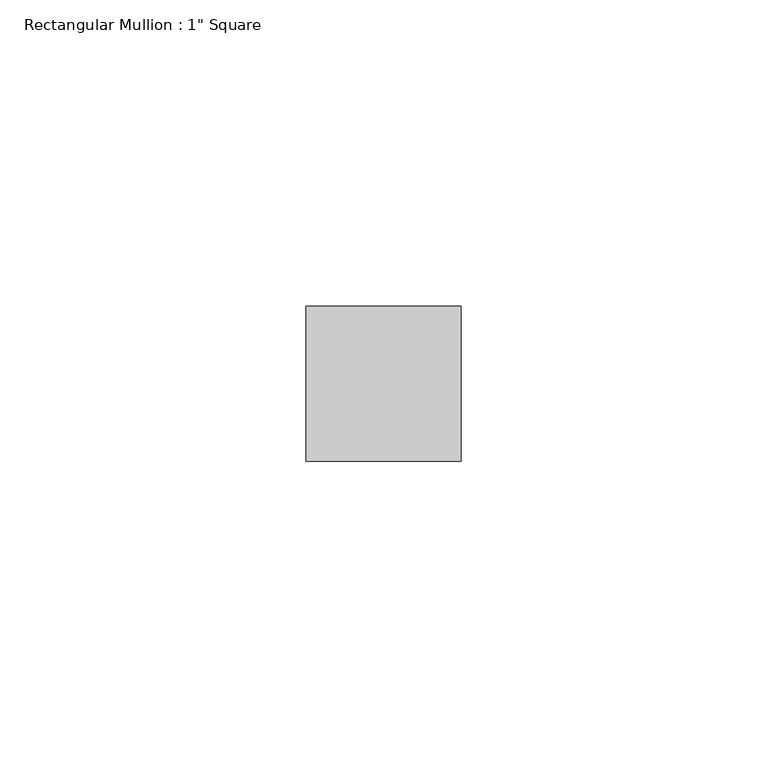
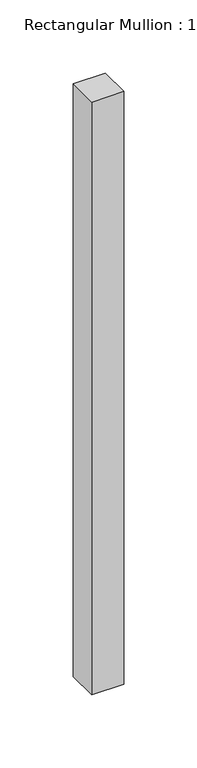
"""IFC4 building model written with IfcOpenShell, lengths in millimetres: member geometry."""

from ifc_helpers import new_model, si_unit, frame, origin, place, context, project, spatial, polyline, outline, extrude, source, transform, mapped, element, save


def member_5ac041f4(model_context):
    return source(origin(), model_context, "Body", "SweptSolid", [
        extrude(outline(polyline([(12.7, 12.7), (12.7, -12.7), (-12.7, -12.7), (-12.7, 12.7), (12.7, 12.7)])), frame((0.0, 0.0, -495.6398623), z_axis=(0.0, 0.0, 1.0), x_axis=(1.0, 0.0, 0.0)), (0.0, 0.0, 1.0), 495.6398623),
    ])


if __name__ == "__main__":
    model = new_model("IFC4")
    model_context = context("Model", 3, world=origin())
    ifc_project = project(units=[si_unit("LENGTHUNIT", "METRE", prefix="MILLI")], contexts=[model_context])
    site = spatial("IfcSite", under=ifc_project)
    building = spatial("IfcBuilding", under=site)
    placement = place(None, origin())
    member_shape = member_5ac041f4(model_context)
    element("IfcMember", 1, ObjectType="Rectangular Mullion : 1\" Square", at=placement, inside=building, context=model_context, shape_type="MappedRepresentation", body=[
        mapped(member_shape, transform((0.0, 0.0, 0.0), x_axis=(1.0, 0.0, 0.0), y_axis=(0.0, 1.0, 0.0), z_axis=(0.0, 0.0, 1.0))),
    ])
    save(model, "model.ifc")

# Revit data of these elements
# Type "Rectangular Mullion : 1\" Square"
#   built-in parameter 1007304 = 0.0833333 (stored number, unit not read)
#   built-in parameter 1007301 = 0.0416667 (stored number, unit not read)
#   built-in parameter 1007300 = 0.0416667 (stored number, unit not read)
